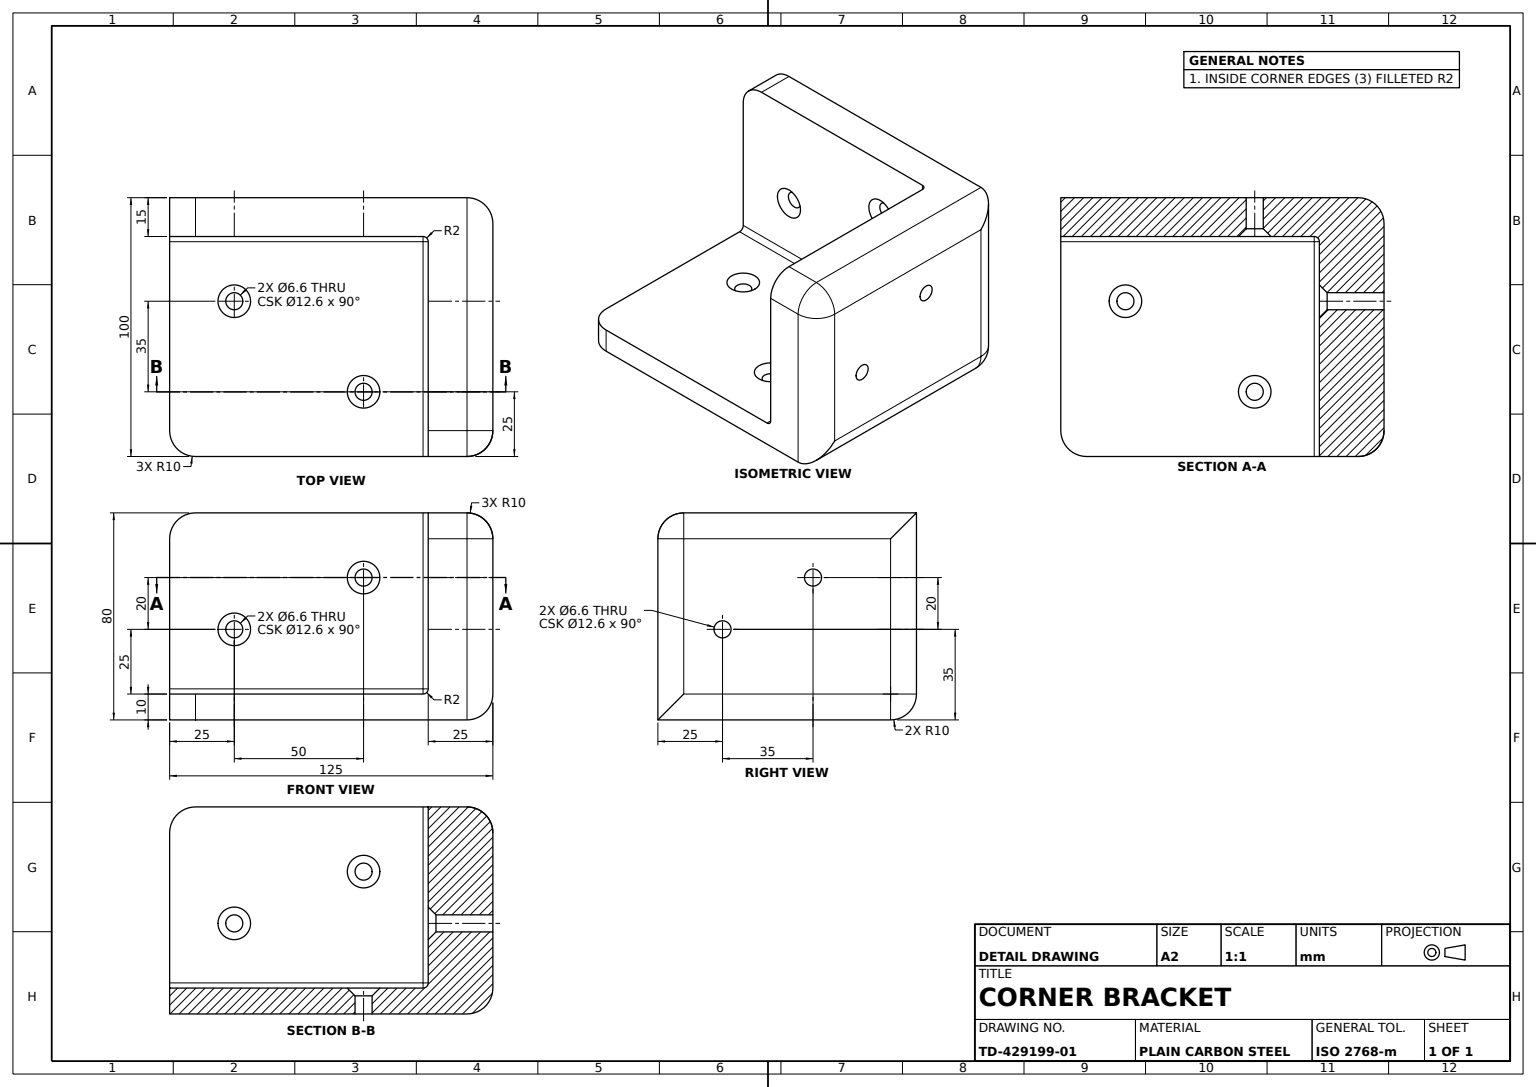
SolidWorks part; units mm, degrees
material "Plain Carbon Steel"
ref_plane "Front Plane" through (0, 0, 0) normal (0, 0, 1) x (1, 0, 0)
ref_plane "Top Plane" through (0, 0, 0) normal (0, 1, 0) x (1, 0, 0)
ref_plane "Right Plane" through (0, 0, 0) normal (1, 0, 0) x (0, 0, -1)
sketch "Bracket L-Profile Sketch" plane through (0, 0, 0) normal (0, 0, 1) x (1, 0, 0)
  line L1 (50, 40) -> (-50, 40)
  line L2 (50, 40) -> (50, -40)
  line L3 (50, -40) -> (-50, -40)
  line L4 (-50, 40) -> (-50, -40)
  line L5 (50, 40) -> (-50, -40) construction
  line L6 (50, -40) -> (-50, 40) construction
  point P0 (0, 0)
  dimension "D1" = 100
  dimension "D2" = 80
extrude "Bracket Body" add sketch "Bracket L-Profile Sketch" along normal blind 125
sketch "Rectangular Cut Sketch 10x15" plane through (0, 0, 125) normal (0, 0, 1) x (1, 0, 0)
  line L0 (-50, -40) -> (50, -40) construction
  line L1 (50, 40) -> (-35, 40)
  line L2 (50, 40) -> (50, -30)
  line L3 (50, -30) -> (-35, -30)
  line L4 (-35, 40) -> (-35, -30)
  line L5 (-50, 40) -> (-50, -40) construction
  dimension "D1" = 10
  dimension "D2" = 15
extrude "Rectangular Cut 10x15" cut sketch "Rectangular Cut Sketch 10x15" against normal offset from surface (100 mm away) 25 up to face at (0, 0, 0)
sketch "CSK Hole Positions Face A" plane through (0, 0, 25) normal (0, 0, 1) x (1, 0, 0)
  line L0 (50, 40) -> (-35, 40) construction
  line L1 (50, -30) -> (50, 40) construction
  point P0 (-10, 15)
  point P1 (25, -5)
  dimension "D1" = 25
  dimension "D2" = 20
  dimension "D3" = 35
  dimension "D4" = 25
sketch "CSK Hole Positions Face B" plane through (-35, 0, 0) normal (1, 0, 0) x (0, 0, -1)
  line L0 (-125, 40) -> (-125, -30) construction
  line L1 (-25, 40) -> (-125, 40) construction
  point P0 (-100, -5)
  point P1 (-50, 15)
  dimension "D1" = 25
  dimension "D2" = 50
  dimension "D3" = 25
  dimension "D4" = 20
sketch "CSK Hole Positions Face C" plane through (0, -30, 0) normal (0, 1, 0) x (1, 0, 0)
  point P0 (-10, -100)
  point P1 (25, -50)
hole_wizard "Countersunk Holes 6xM6" positions "3DSketch1" profile "Sketch7" countersink size "M6" standard "ANSI Metric"
sketch3d "3DSketch1"
  point P0 (-35, -5, 100)
  point P3 (-35, 15, 50)
  point P6 (-10, -30, 100)
  point P9 (25, -30, 50)
  point P12 (25, -5, 25)
  point P15 (-10, 15, 25)
sketch "Sketch7" plane through (-35, -5, 100) normal (0, 1, 0) x (0, 0, -1)
  line L0 (0, 0) -> (0, 38)
  line L1 (0, 38) -> (3.3, 36.0172)
  line L2 (3.3, 36.0172) -> (3.3, 3)
  line L3 (3.3, 3) -> (6.3, 0)
  line L5 (6.3, 0) -> (0, 0)
  line L6 (-3.3, 3) -> (-6.3, 0) construction
  line L10 (0, 38) -> (-3.3, 36.0172) construction
  line L11 (0, -6.35) -> (0, 107.95) construction
  dimension "Hole Dia." = 6.6
  dimension "Hole Depth" = 38
  dimension "Near C'Sink Dia." = 12.6
  dimension "Near C'Sink Angle" = 90
  dimension "Drill Angle" = 118
fillet "Outer Edge Fillets R10" radius 10 8 edges at (50, -35, 125) (0, 40, 0) (-50, 0, 0) (0, -40, 0) (50, 0, 0) (50, 40, 12.5) (-42.5, 40, 125) (-50, -40, 62.5)
fillet "Edge Fillets R2" radius 2 3 edges at (7.5, -30, 25) (-35, 5, 25) (-35, -30, 75)
